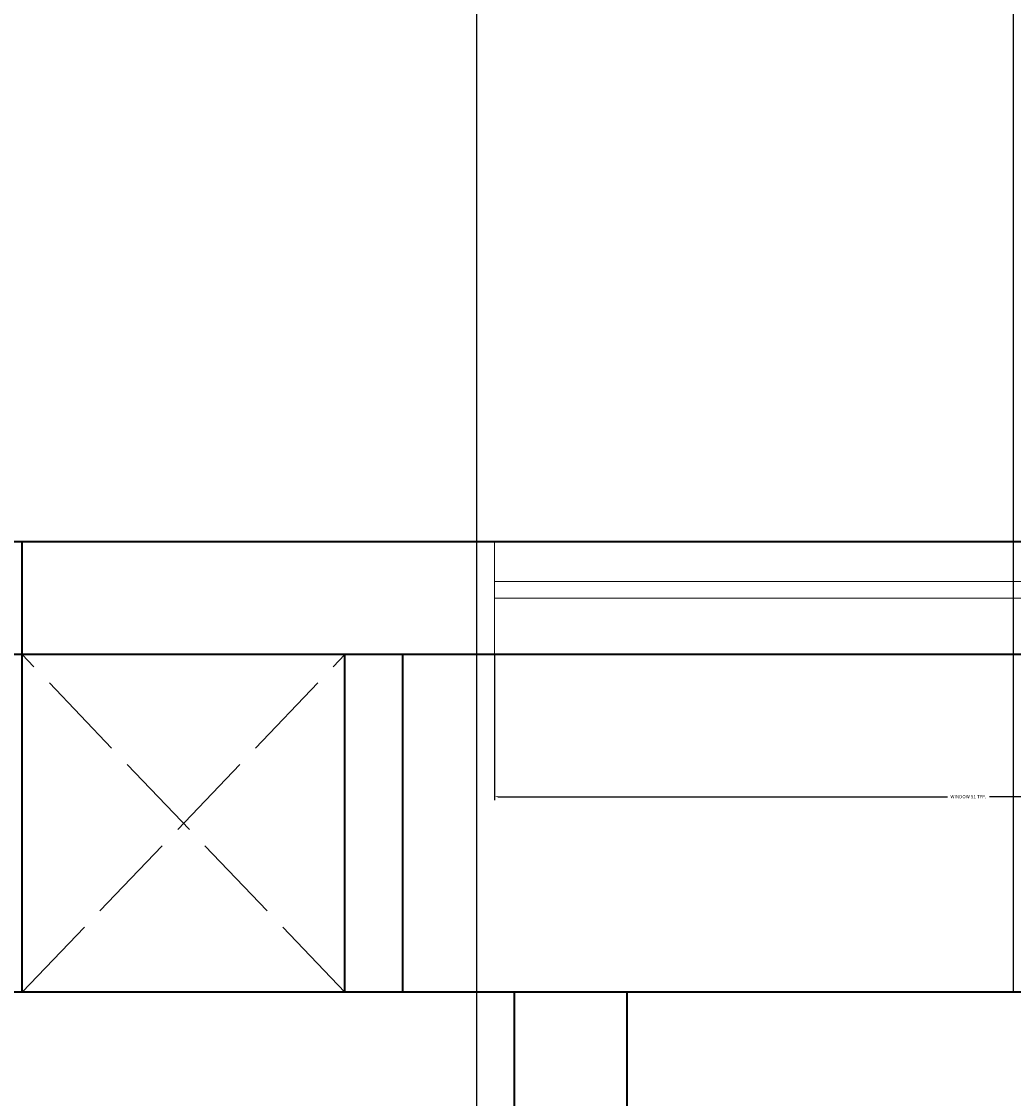
# Model space of a CAD drawing. Units: inches. Extents: x -61 to 1599, y -1316 to 257.
# Tile 72 of 204: x 295 to 348, y -623 to -565. Entities that reach past the tile are written whole.
import ezdxf

# ---------------------------------------------------------------- set-up
doc = ezdxf.new("R2010")
doc.units = ezdxf.units.IN
doc.header["$MEASUREMENT"] = 0
doc.linetypes.add('ACAD_ISO02W100', pattern=[15, 12, -3])
for name, color, linetype, lineweight in [('A-ANNO-DIMS', 2, 'Continuous', 18), ('A-FLOR-OPEN-HIDN', 8, 'ACAD_ISO02W100', 13), ('WALLS', 4, 'Continuous', 35), ('WINDOWS', 220, 'Continuous', 18)]:
    doc.layers.add(name, color=color, linetype=linetype, lineweight=lineweight)
doc.styles.get("Standard").update_dxf_attribs({"font": 'arial.ttf'})
doc.dimstyles.get("Standard").update_dxf_attribs({"dimtxt": 0.18, "dimasz": 0.18, "dimexe": 0.18, "dimexo": 0.0625, "dimgap": 0.09, "dimtad": 0, "dimtih": 1, "dimtoh": 1, "dimdec": 0, "dimzin": 0, "dimdsep": 46, "dimlunit": 3, "dimtxsty": 'Standard', "dimcen": 0.09, "dimadec": 0, "dimazin": 0, "dimtfac": 1, "dimtdec": 0, "dimtofl": 0, "dimtmove": 0, "dimatfit": 3, "dimfxl": 1, "dimtolj": 1, "dimtzin": 0, "dimarcsym": 0})

# ---------------------------------------------------------------- blocks, each defined once
blk = doc.blocks.new('WIN-51IN')
for p, q in [((0, 0), (0, 6)), ((50.516, 0), (50.516, 6)), ((0, 3.885), (50.516, 3.885)), ((0, 3), (50.516, 3))]:
    blk.add_line(p, q)
blk = doc.blocks.new('*D642')
at = {"layer": 'A-ANNO-DIMS', "color": 0, "lineweight": -2, "transparency": 16777216}
for p, q in [((320.659, -599.007), (320.659, -606.702)), ((371.175, -599.007), (371.175, -606.702)), ((320.839, -606.522), (344.798, -606.522)), ((370.995, -606.522), (347.035, -606.522))]:
    blk.add_line(p, q, dxfattribs=at)
at = {"layer": 'A-ANNO-DIMS', "color": 0, "transparency": 16777216}
for points in [[(320.839, -606.492), (320.839, -606.552), (320.659, -606.522)], [(370.995, -606.492), (370.995, -606.552), (371.175, -606.522)]]:
    blk.add_solid(points, dxfattribs=at)
at = {"layer": 'DEFPOINTS', "color": 0, "transparency": 16777216}
for p in [(320.659, -598.945), (371.175, -598.945), (371.175, -606.522)]:
    blk.add_point(p, dxfattribs=at)
at = {"layer": 'A-ANNO-DIMS', "color": 0, "transparency": 16777216, "insert": (345.917, -606.522), "char_height": 0.18, "attachment_point": 5}
blk.add_mtext('\\A1;WINDOW 51 TYP.', dxfattribs=at)
blk = doc.blocks.new('*D687')
at = {"layer": 'A-ANNO-DIMS', "color": 0, "lineweight": -2, "transparency": 16777216}
for p, q in [((289.418, 181.677), (-61.077, 181.677)), ((-60.897, 181.497), (-60.897, -528.952)), ((-60.897, -1239.765), (-60.897, -529.316)), ((319.64, -1239.945), (-61.077, -1239.945))]:
    blk.add_line(p, q, dxfattribs=at)
at = {"layer": 'A-ANNO-DIMS', "color": 0, "transparency": 16777216}
for points in [[(-60.927, 181.497), (-60.867, 181.497), (-60.897, 181.677)], [(-60.927, -1239.765), (-60.867, -1239.765), (-60.897, -1239.945)]]:
    blk.add_solid(points, dxfattribs=at)
at = {"layer": 'DEFPOINTS', "color": 0, "transparency": 16777216}
for p in [(289.481, 181.677), (-60.897, -1239.945), (319.703, -1239.945)]:
    blk.add_point(p, dxfattribs=at)
at = {"layer": 'A-ANNO-DIMS', "color": 0, "transparency": 16777216, "insert": (-60.897, -529.134), "char_height": 0.18, "attachment_point": 5}
blk.add_mtext('\\A1;1421.6', dxfattribs=at)
blk = doc.blocks.new('*D702')
at = {"layer": 'A-ANNO-DIMS', "color": 0, "lineweight": -2, "transparency": 16777216}
for p, q in [((276.882, -616.882), (276.882, 257.457)), ((277.062, 257.277), (312.209, 257.277)), ((348.14, 257.277), (312.994, 257.277)), ((348.32, -616.882), (348.32, 257.457))]:
    blk.add_line(p, q, dxfattribs=at)
at = {"layer": 'A-ANNO-DIMS', "color": 0, "transparency": 16777216}
for points in [[(277.062, 257.307), (277.062, 257.247), (276.882, 257.277)], [(348.14, 257.307), (348.14, 257.247), (348.32, 257.277)]]:
    blk.add_solid(points, dxfattribs=at)
at = {"layer": 'DEFPOINTS', "color": 0, "transparency": 16777216}
for p in [(348.32, 257.277), (276.882, -616.945), (348.32, -616.945)]:
    blk.add_point(p, dxfattribs=at)
at = {"layer": 'A-ANNO-DIMS', "color": 0, "transparency": 16777216, "insert": (312.601, 257.277), "char_height": 0.18, "attachment_point": 5}
blk.add_mtext('\\A1;71.44', dxfattribs=at)
blk = doc.blocks.new('*D710')
at = {"layer": 'A-ANNO-DIMS', "color": 0, "lineweight": -2, "transparency": 16777216}
for p, q in [((319.703, -465.385), (319.703, -1315.725)), ((403.703, -465.385), (403.703, -1315.725)), ((319.883, -1315.545), (361.484, -1315.545)), ((403.523, -1315.545), (361.921, -1315.545))]:
    blk.add_line(p, q, dxfattribs=at)
at = {"layer": 'A-ANNO-DIMS', "color": 0, "transparency": 16777216}
for points in [[(319.883, -1315.515), (319.883, -1315.575), (319.703, -1315.545)], [(403.523, -1315.515), (403.523, -1315.575), (403.703, -1315.545)]]:
    blk.add_solid(points, dxfattribs=at)
at = {"layer": 'DEFPOINTS', "color": 0, "transparency": 16777216}
for p in [(319.703, -465.323), (403.703, -465.323), (403.703, -1315.545)]:
    blk.add_point(p, dxfattribs=at)
at = {"layer": 'A-ANNO-DIMS', "color": 0, "transparency": 16777216, "insert": (361.703, -1315.545), "char_height": 0.18, "attachment_point": 5}
blk.add_mtext('\\A1;84', dxfattribs=at)

msp = doc.modelspace()

# ---------------------------------------------------------------- linework, layer by layer
at = {"layer": 'A-FLOR-OPEN-HIDN', "ltscale": 0.4}
for p, q in [((295.4807, -616.9446), (312.6819, -598.9446)), ((312.6819, -616.9446), (295.4807, -598.9446))]:
    msp.add_line(p, q, dxfattribs=at)
at = {"layer": 'WALLS'}
for p, q in [((403.7028, -592.9446), (289.4807, -592.9446)), ((295.4807, -616.9446), (295.4807, -592.9446)), ((403.7028, -598.9446), (289.4807, -598.9446)), ((312.6819, -616.9446), (312.6819, -598.9446)), ((315.7747, -616.9446), (315.7747, -598.9446)), ((544.7028, -616.9446), (14.7028, -616.9446)), ((321.7028, -616.9446), (321.7028, -787.9446)), ((327.7028, -616.9446), (327.7028, -787.9446))]:
    msp.add_line(p, q, dxfattribs=at)

# ---------------------------------------------------------------- block references
at = {"layer": 'WINDOWS'}
msp.add_blockref('WIN-51IN', (320.659, -598.9447), dxfattribs=at)

# ---------------------------------------------------------------- dimensions: what is measured, and where the dimension line sits
at = {"layer": 'A-ANNO-DIMS'}
for base, p1, p2, override, picture, middle in [((348.3201, 257.2771), (276.8825, -616.9446), (348.3201, -616.9446), {"dimdec": 2, "dimlfac": 1, "dimrnd": 0, "dimzin": 0, "dimdsep": 46, "dimlunit": 2}, '*D702', (312.6013, 257.2771)), ((403.7028, -1315.5446), (319.7028, -465.3229), (403.7028, -465.3229), {"dimdec": 0, "dimlfac": 1, "dimrnd": 0, "dimzin": 0, "dimdsep": 46, "dimlunit": 2}, '*D710', (361.7028, -1315.5446))]:
    dim = msp.add_linear_dim(base=base, p1=p1, p2=p2, dimstyle='Standard', override=override, dxfattribs=at)
    dim.commit()
    dim.dimension.update_dxf_attribs({"geometry": picture, "text_midpoint": middle})
dim = msp.add_linear_dim(base=(-60.8972, -1239.9446), p1=(289.4807, 181.6771), p2=(319.7028, -1239.9446), angle=90, dimstyle='Standard', override={"dimdec": 1, "dimlfac": 1, "dimrnd": 0, "dimzin": 0, "dimdsep": 46, "dimlunit": 2}, dxfattribs=at)
dim.commit()
dim.dimension.update_dxf_attribs({"geometry": '*D687', "text_midpoint": (-60.8972, -529.1337)})
dim = msp.add_linear_dim(base=(371.1745, -606.5219), p1=(320.659, -598.9446), p2=(371.1745, -598.9446), text='WINDOW <> TYP.', dimstyle='Standard', override={"dimdec": 0, "dimlfac": 1, "dimrnd": 0, "dimzin": 0, "dimdsep": 46, "dimlunit": 2}, dxfattribs=at)
dim.commit()
dim.dimension.update_dxf_attribs({"geometry": '*D642', "text_midpoint": (345.9168, -606.5219)})

doc.saveas('drawing.dxf')
